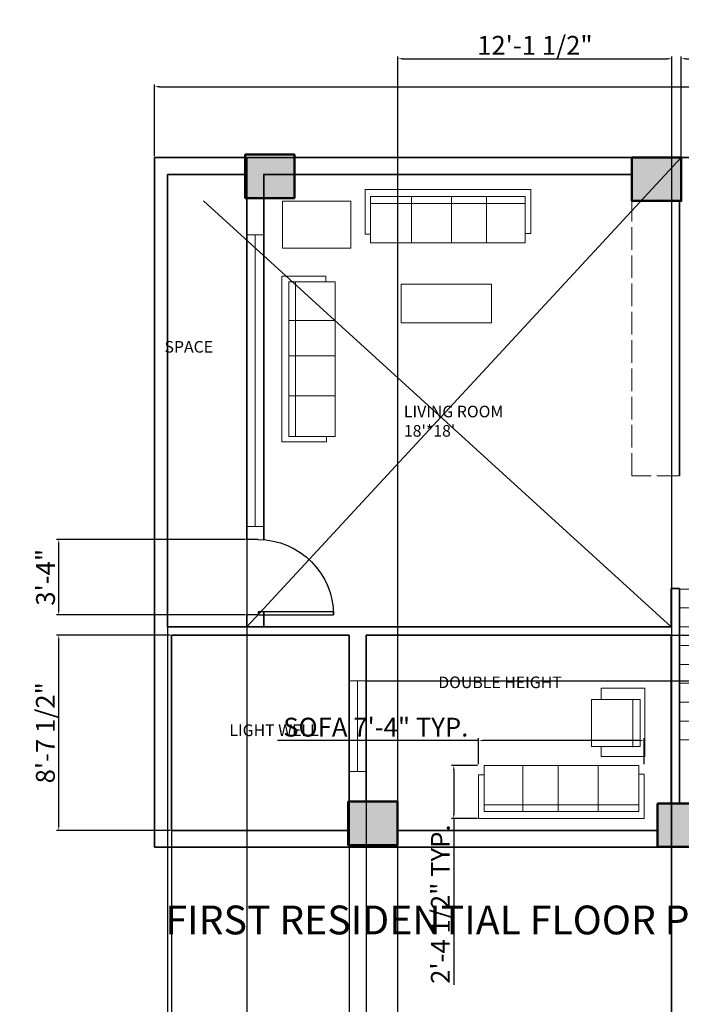
# Model space of a CAD drawing. Units: inches. Extents: x 1964 to 3462, y 1879 to 2909.
# Tile 3 of 4: x 2631 to 2982, y 2387 to 2909. Entities that reach past the tile are written whole.
import ezdxf

# ---------------------------------------------------------------- set-up
doc = ezdxf.new("R2010")
doc.units = ezdxf.units.IN
doc.linetypes.add('ACAD_ISO02W100', pattern=[15, 12, -3])
for name, color, linetype, lineweight in [('A-ANNO-DIMS', 2, 'Continuous', 18), ('A-ANNO-TEXT', 7, 'Continuous', 35), ('A-AREA-IDEN', 7, 'Continuous', 18), ('A-COLS', 1, 'Continuous', 50), ('A-COLS-PATT', 252, 'Continuous', 13), ('A-DOOR', 4, 'Continuous', 25), ('A-FLOR-OPEN', 8, 'Continuous', 13), ('A-FLOR-OVHD', 8, 'ACAD_ISO02W100', 18), ('A-FLOR-STRS', 3, 'Continuous', 18), ('A-FURN', 8, 'Continuous', 18), ('A-GLAZ', 4, 'Continuous', 18), ('A-WALL', 7, 'Continuous', 35)]:
    doc.layers.add(name, color=color, linetype=linetype, lineweight=lineweight)
doc.styles.get("Standard").update_dxf_attribs({"font": 'arial.ttf'})
doc.dimstyles.new('ISO-25', dxfattribs={"dimtxt": 10, "dimasz": 2.5, "dimexe": 1.25, "dimexo": 0.625, "dimtad": 1, "dimdec": 0, "dimlunit": 4, "dimtxsty": 'Standard', "dimcen": 2.5, "dimadec": 0, "dimazin": 0, "dimtfac": 1, "dimtdec": 0, "dimtmove": 0, "dimatfit": 3, "dimfxl": 1, "dimarcsym": 0})

# ---------------------------------------------------------------- blocks, each defined once
blk = doc.blocks.new('*U2')
for p, q in [((0, 0), (0, -6)), ((40, 0), (40, -6))]:
    blk.add_line(p, q)
blk.add_lwpolyline([(0, 0), (0, 40), (1.75, 40), (1.75, 0)], close=True)
blk.add_arc((0, 0), 40, 0, 90)
blk = doc.blocks.new('*D9')
at = {"layer": 'A-ANNO-DIMS', "color": 0, "lineweight": -2, "transparency": 16777216}
for p, q in [((2702.98, 2836.98), (2702.98, 2875.1)), ((2705.48, 2873.85), (3378.17, 2873.85)), ((3380.67, 2836.98), (3380.67, 2875.1))]:
    blk.add_line(p, q, dxfattribs=at)
at = {"layer": 'A-ANNO-DIMS', "color": 0, "lineweight": 100, "transparency": 16777216}
for points in [[(2705.48, 2874.26), (2705.48, 2873.43), (2702.98, 2873.85)], [(3378.17, 2874.26), (3378.17, 2873.43), (3380.67, 2873.85)]]:
    blk.add_solid(points, dxfattribs=at)
at = {"layer": 'Defpoints', "color": 0, "lineweight": 100, "transparency": 16777216}
for p in [(3380.67, 2873.85), (2702.98, 2836.36), (3380.67, 2836.36)]:
    blk.add_point(p, dxfattribs=at)
at = {"layer": 'A-ANNO-DIMS', "color": 0, "transparency": 16777216, "insert": (3041.82, 2879.58), "char_height": 10, "attachment_point": 5}
blk.add_mtext('56\'-6"', dxfattribs=at)
blk = doc.blocks.new('COL-RECT-26x23')
blk.add_lwpolyline([(0, 23.08), (26.15, 23.08), (26.15, 0), (0, 0)], close=True)
blk = doc.blocks.new('SOFA-4SEAT')
for p, q in [((0, 4.61), (0, 28.28)), ((0, 28.28), (87.86, 28.28)), ((87.86, 4.94), (87.86, 28.28)), ((2.86, 20.93), (84.86, 20.93)), ((24.5, 24.53), (24.5, 0)), ((45.74, 24.53), (45.74, 0)), ((64.36, 24.53), (64.36, 0)), ((2.86, 4.61), (0, 4.61)), ((84.86, 4.94), (87.86, 4.94))]:
    blk.add_line(p, q)
blk.add_lwpolyline([(2.86, 24.53), (84.86, 24.53), (84.86, 0), (2.86, 0)], close=True)
blk = doc.blocks.new('STAIR-RETURN-RESIDENTIAL')
for p, q in [((0, 128), (145.76, 128)), ((21.08, 128), (15.66, 121.5)), ((21.08, 21.87), (21.08, 128)), ((21.08, 128), (26.5, 121.5)), ((43.5, 124.05), (43.5, 128)), ((97.76, 128), (97.76, 118)), ((119.78, 128), (119.78, 21.87)), ((43.5, 48), (43.5, 124.05)), ((47.14, 51.64), (47.14, 120.41)), ((47.14, 120.41), (94.12, 120.41)), ((94.12, 51.64), (94.12, 120.41)), ((97.76, 48), (97.76, 124.05)), ((0, 118), (43.5, 118)), ((97.76, 118), (145.76, 118)), ((0, 108), (43.5, 108)), ((97.76, 108), (145.76, 108)), ((0, 98), (43.5, 98)), ((97.76, 98), (145.76, 98)), ((0, 88), (43.5, 88)), ((97.76, 88), (145.76, 88)), ((0, 78), (43.5, 78)), ((97.76, 78), (145.76, 78)), ((0, 68), (43.5, 68)), ((97.76, 68), (145.76, 68)), ((0, 58), (43.5, 58)), ((97.76, 58), (145.76, 58)), ((0, 48), (145.76, 48)), ((97.76, 48), (43.5, 48)), ((43.5, 48), (43.5, 0)), ((94.12, 51.64), (47.14, 51.64)), ((53.5, 48), (53.5, 0)), ((63.5, 48), (63.5, 0)), ((73.5, 48), (73.5, 0)), ((83.5, 48), (83.5, 0)), ((97.76, 50.18), (97.76, 0)), ((119.78, 21.87), (21.08, 21.87))]:
    blk.add_line(p, q)
blk = doc.blocks.new('WIN-48IN')
blk.add_line((4.5, 0), (4.5, 48.18))
blk.add_lwpolyline([(0, 0), (9, 0), (9, 48.18), (0, 48.18)], close=True)
blk = doc.blocks.new('*D25')
at = {"layer": 'A-ANNO-DIMS', "color": 0, "lineweight": -2, "transparency": 16777216}
for p, q in [((2874.86, 2514.46), (2874.86, 2528.27)), ((2962.72, 2514.46), (2962.72, 2528.27)), ((2874.86, 2527.02), (2768.29, 2527.02)), ((2960.22, 2527.02), (2877.36, 2527.02))]:
    blk.add_line(p, q, dxfattribs=at)
at = {"layer": 'A-ANNO-DIMS', "color": 0, "lineweight": 100, "transparency": 16777216}
for points in [[(2877.36, 2527.43), (2877.36, 2526.6), (2874.86, 2527.02)], [(2960.22, 2527.43), (2960.22, 2526.6), (2962.72, 2527.02)]]:
    blk.add_solid(points, dxfattribs=at)
at = {"layer": 'Defpoints', "color": 0, "lineweight": 100, "transparency": 16777216}
for p in [(2874.86, 2527.02), (2874.86, 2513.84), (2962.72, 2513.84)]:
    blk.add_point(p, dxfattribs=at)
at = {"layer": 'A-ANNO-DIMS', "color": 0, "transparency": 16777216, "insert": (2820.33, 2532.81), "char_height": 10, "attachment_point": 5}
blk.add_mtext('SOFA 7\'-4" TYP.', dxfattribs=at)
blk = doc.blocks.new('*D26')
at = {"layer": 'A-ANNO-DIMS', "color": 0, "lineweight": -2, "transparency": 16777216}
for p, q in [((2874.24, 2513.84), (2860.44, 2513.84)), ((2861.69, 2511.34), (2861.69, 2488.06)), ((2874.24, 2485.56), (2860.44, 2485.56)), ((2861.69, 2485.56), (2861.69, 2397.38))]:
    blk.add_line(p, q, dxfattribs=at)
at = {"layer": 'A-ANNO-DIMS', "color": 0, "lineweight": 100, "transparency": 16777216}
for points in [[(2861.27, 2511.34), (2862.1, 2511.34), (2861.69, 2513.84)], [(2861.27, 2488.06), (2862.1, 2488.06), (2861.69, 2485.56)]]:
    blk.add_solid(points, dxfattribs=at)
at = {"layer": 'Defpoints', "color": 0, "lineweight": 100, "transparency": 16777216}
for p in [(2874.86, 2513.84), (2861.69, 2485.56), (2874.86, 2485.56)]:
    blk.add_point(p, dxfattribs=at)
at = {"layer": 'A-ANNO-DIMS', "color": 0, "transparency": 16777216, "insert": (2855.89, 2440.22), "char_height": 10, "attachment_point": 5, "rotation": 90}
blk.add_mtext('2\'-4 1/2" TYP.', dxfattribs=at)
blk = doc.blocks.new('*D53')
at = {"layer": 'A-ANNO-DIMS', "color": 0, "lineweight": -2, "transparency": 16777216}
for p, q in [((2709.93, 2826.73), (2709.93, 1887.22)), ((2751.91, 2826.73), (2751.91, 1887.22)), ((2712.43, 1888.47), (2749.41, 1888.47))]:
    blk.add_line(p, q, dxfattribs=at)
at = {"layer": 'A-ANNO-DIMS', "color": 0, "lineweight": 100, "transparency": 16777216}
for points in [[(2712.43, 1888.89), (2712.43, 1888.06), (2709.93, 1888.47)], [(2749.41, 1888.89), (2749.41, 1888.06), (2751.91, 1888.47)]]:
    blk.add_solid(points, dxfattribs=at)
at = {"layer": 'Defpoints', "color": 0, "lineweight": 100, "transparency": 16777216}
for p in [(2709.93, 2827.36), (2751.91, 2827.36), (2751.91, 1888.47)]:
    blk.add_point(p, dxfattribs=at)
at = {"layer": 'A-ANNO-DIMS', "color": 0, "transparency": 16777216, "insert": (2730.92, 1894.21), "char_height": 10, "attachment_point": 5}
blk.add_mtext('3\'-6"', dxfattribs=at)
blk = doc.blocks.new('*D54')
at = {"layer": 'A-ANNO-DIMS', "color": 0, "lineweight": -2, "transparency": 16777216}
for p, q in [((2751.29, 2633.6), (2650.93, 2633.6)), ((2652.18, 2596.1), (2652.18, 2631.1)), ((2751.29, 2593.6), (2650.93, 2593.6))]:
    blk.add_line(p, q, dxfattribs=at)
at = {"layer": 'A-ANNO-DIMS', "color": 0, "lineweight": 100, "transparency": 16777216}
for points in [[(2651.76, 2631.1), (2652.59, 2631.1), (2652.18, 2633.6)], [(2651.76, 2596.1), (2652.59, 2596.1), (2652.18, 2593.6)]]:
    blk.add_solid(points, dxfattribs=at)
at = {"layer": 'Defpoints', "color": 0, "lineweight": 100, "transparency": 16777216}
for p in [(2652.18, 2633.6), (2751.91, 2633.6), (2751.91, 2593.6)]:
    blk.add_point(p, dxfattribs=at)
at = {"layer": 'A-ANNO-DIMS', "color": 0, "transparency": 16777216, "insert": (2646.44, 2613.6), "char_height": 10, "attachment_point": 5, "rotation": 90}
blk.add_mtext('3\'-4"', dxfattribs=at)
blk = doc.blocks.new('*D55')
at = {"layer": 'A-ANNO-DIMS', "color": 0, "lineweight": -2, "transparency": 16777216}
for p, q in [((2982.37, 2813.9), (2982.37, 2889.94)), ((2984.87, 2888.69), (3166.19, 2888.69)), ((3168.69, 2813.9), (3168.69, 2889.94))]:
    blk.add_line(p, q, dxfattribs=at)
at = {"layer": 'A-ANNO-DIMS', "color": 0, "lineweight": 100, "transparency": 16777216}
for points in [[(2984.87, 2889.1), (2984.87, 2888.27), (2982.37, 2888.69)], [(3166.19, 2889.1), (3166.19, 2888.27), (3168.69, 2888.69)]]:
    blk.add_solid(points, dxfattribs=at)
at = {"layer": 'Defpoints', "color": 0, "lineweight": 100, "transparency": 16777216}
for p in [(3168.69, 2888.69), (2982.37, 2813.28), (3168.69, 2813.28)]:
    blk.add_point(p, dxfattribs=at)
at = {"layer": 'A-ANNO-DIMS', "color": 0, "transparency": 16777216, "insert": (3075.53, 2894.48), "char_height": 10, "attachment_point": 5}
blk.add_mtext('15\'-6 1/2"', dxfattribs=at)
blk = doc.blocks.new('*D57')
at = {"layer": 'A-ANNO-DIMS', "color": 0, "lineweight": -2, "transparency": 16777216}
for p, q in [((2711.98, 2582.23), (2711.98, 1887.22)), ((2806.18, 2582.23), (2806.18, 1887.22)), ((2714.48, 1888.47), (2803.68, 1888.47))]:
    blk.add_line(p, q, dxfattribs=at)
at = {"layer": 'A-ANNO-DIMS', "color": 0, "lineweight": 100, "transparency": 16777216}
for points in [[(2714.48, 1888.89), (2714.48, 1888.06), (2711.98, 1888.47)], [(2803.68, 1888.89), (2803.68, 1888.06), (2806.18, 1888.47)]]:
    blk.add_solid(points, dxfattribs=at)
at = {"layer": 'Defpoints', "color": 0, "lineweight": 100, "transparency": 16777216}
for p in [(2711.98, 2582.86), (2806.18, 2582.86), (2806.18, 1888.47)]:
    blk.add_point(p, dxfattribs=at)
at = {"layer": 'A-ANNO-DIMS', "color": 0, "transparency": 16777216, "insert": (2759.08, 1894.2), "char_height": 10, "attachment_point": 5}
blk.add_mtext('7\'-10"', dxfattribs=at)
blk = doc.blocks.new('*D58')
at = {"layer": 'A-ANNO-DIMS', "color": 0, "lineweight": -2, "transparency": 16777216}
for p, q in [((2815.18, 2582.23), (2815.18, 1887.22)), ((2976.91, 2582.23), (2976.91, 1887.22)), ((2817.68, 1888.47), (2974.41, 1888.47))]:
    blk.add_line(p, q, dxfattribs=at)
at = {"layer": 'A-ANNO-DIMS', "color": 0, "lineweight": 100, "transparency": 16777216}
for points in [[(2817.68, 1888.89), (2817.68, 1888.06), (2815.18, 1888.47)], [(2974.41, 1888.89), (2974.41, 1888.06), (2976.91, 1888.47)]]:
    blk.add_solid(points, dxfattribs=at)
at = {"layer": 'Defpoints', "color": 0, "lineweight": 100, "transparency": 16777216}
for p in [(2815.18, 2582.86), (2976.91, 2582.86), (2976.91, 1888.47)]:
    blk.add_point(p, dxfattribs=at)
at = {"layer": 'A-ANNO-DIMS', "color": 0, "transparency": 16777216, "insert": (2896.05, 1894.27), "char_height": 10, "attachment_point": 5}
blk.add_mtext('13\'-5 1/2"', dxfattribs=at)
blk = doc.blocks.new('*D59')
at = {"layer": 'A-ANNO-DIMS', "color": 0, "lineweight": -2, "transparency": 16777216}
for p, q in [((2711.35, 2582.86), (2650.93, 2582.86)), ((2652.18, 2481.86), (2652.18, 2580.36)), ((2711.35, 2479.36), (2650.93, 2479.36))]:
    blk.add_line(p, q, dxfattribs=at)
at = {"layer": 'A-ANNO-DIMS', "color": 0, "lineweight": 100, "transparency": 16777216}
for points in [[(2651.76, 2580.36), (2652.59, 2580.36), (2652.18, 2582.86)], [(2651.76, 2481.86), (2652.59, 2481.86), (2652.18, 2479.36)]]:
    blk.add_solid(points, dxfattribs=at)
at = {"layer": 'Defpoints', "color": 0, "lineweight": 100, "transparency": 16777216}
for p in [(2652.18, 2582.86), (2711.98, 2582.86), (2711.98, 2479.36)]:
    blk.add_point(p, dxfattribs=at)
at = {"layer": 'A-ANNO-DIMS', "color": 0, "transparency": 16777216, "insert": (2646.38, 2531.11), "char_height": 10, "attachment_point": 5, "rotation": 90}
blk.add_mtext('8\'-7 1/2"', dxfattribs=at)
blk = doc.blocks.new('*D60')
at = {"layer": 'A-ANNO-DIMS', "color": 0, "lineweight": -2, "transparency": 16777216}
for p, q in [((3448.35, 2582.86), (3448.35, 2613.36)), ((2815.81, 2582.86), (3449.6, 2582.86)), ((3448.35, 2561.25), (3448.35, 2580.36)), ((2815.81, 2558.75), (3449.6, 2558.75))]:
    blk.add_line(p, q, dxfattribs=at)
at = {"layer": 'A-ANNO-DIMS', "color": 0, "lineweight": 100, "transparency": 16777216}
for points in [[(3447.94, 2580.36), (3448.77, 2580.36), (3448.35, 2582.86)], [(3447.94, 2561.25), (3448.77, 2561.25), (3448.35, 2558.75)]]:
    blk.add_solid(points, dxfattribs=at)
at = {"layer": 'Defpoints', "color": 0, "lineweight": 100, "transparency": 16777216}
for p in [(2815.18, 2582.86), (3448.35, 2582.86), (2815.18, 2558.75)]:
    blk.add_point(p, dxfattribs=at)
at = {"layer": 'A-ANNO-DIMS', "color": 0, "transparency": 16777216, "insert": (3442.62, 2599.36), "char_height": 10, "attachment_point": 5, "rotation": 90}
blk.add_mtext('2\'-0"', dxfattribs=at)
blk = doc.blocks.new('*D64')
at = {"layer": 'A-ANNO-DIMS', "color": 0, "lineweight": -2, "transparency": 16777216}
for p, q in [((2832.07, 2298.2), (2832.07, 2889.94)), ((2834.57, 2888.69), (2974.84, 2888.69)), ((2977.34, 2298.34), (2977.34, 2889.94))]:
    blk.add_line(p, q, dxfattribs=at)
at = {"layer": 'A-ANNO-DIMS', "color": 0, "lineweight": 100, "transparency": 16777216}
for points in [[(2834.57, 2889.1), (2834.57, 2888.27), (2832.07, 2888.69)], [(2974.84, 2889.1), (2974.84, 2888.27), (2977.34, 2888.69)]]:
    blk.add_solid(points, dxfattribs=at)
at = {"layer": 'Defpoints', "color": 0, "lineweight": 100, "transparency": 16777216}
for p in [(2977.34, 2888.69), (2832.07, 2297.57), (2977.34, 2297.71)]:
    blk.add_point(p, dxfattribs=at)
at = {"layer": 'A-ANNO-DIMS', "color": 0, "transparency": 16777216, "insert": (2904.7, 2894.48), "char_height": 10, "attachment_point": 5}
blk.add_mtext('12\'-1 1/2"', dxfattribs=at)

msp = doc.modelspace()

# ---------------------------------------------------------------- hatches: boundary and pattern name
at = {"layer": 'A-COLS-PATT'}
h = msp.add_hatch(color=256, dxfattribs=at)
h.dxf.hatch_style = 1
h.paths.add_polyline_path([(2777.22, 2827.36), (2760.91, 2827.36), (2760.91, 2814.8), (2777.22, 2814.8)], flags=17)
h.paths.add_polyline_path([(2777.22, 2836.36), (2751.91, 2836.36), (2751.91, 2814.8), (2760.91, 2814.8), (2760.91, 2827.36), (2777.22, 2827.36)])
h = msp.add_hatch(color=256, dxfattribs=at)
h.dxf.hatch_style = 1
h.paths.add_polyline_path([(3380.67, 2836.36), (3354.52, 2836.36), (3354.52, 2813.28), (3380.67, 2813.28)])
h.paths.add_polyline_path([(3194.85, 2836.36), (3168.69, 2836.36), (3168.69, 2827.36), (3168.91, 2827.36), (3168.91, 2813.28), (3194.85, 2813.28)])
h.paths.add_polyline_path([(2982.37, 2836.36), (2956.21, 2836.36), (2956.21, 2813.28), (2961, 2813.28)])
h.paths.add_polyline_path([(2982.37, 2836.36), (2961, 2813.28), (2981.41, 2813.28), (2982.37, 2813.28)], flags=17)
h.paths.add_polyline_path([(2831.78, 2494.67), (2805.62, 2494.67), (2805.62, 2471.58), (2831.78, 2471.58)])
h.paths.add_polyline_path([(2995.98, 2493.63), (2969.83, 2493.63), (2969.83, 2470.55), (2995.98, 2470.55)])
h.paths.add_polyline_path([(3252.83, 2493.16), (3226.67, 2493.16), (3226.67, 2470.36), (3252.83, 2470.36)])
h.paths.add_polyline_path([(3380.67, 2492.15), (3354.52, 2492.15), (3354.52, 2470.36), (3380.67, 2470.36)])

# ---------------------------------------------------------------- linework, layer by layer
at = {"layer": 'A-FLOR-OPEN'}
for p, q in [((2751.91, 2587.36), (2982.37, 2836.36)), ((2976.91, 2587.36), (2728.87, 2813.28))]:
    msp.add_line(p, q, dxfattribs=at)
at = {"layer": 'A-FLOR-OVHD'}
msp.add_lwpolyline([(2956.21, 2813.28), (2981.41, 2813.28), (2981.41, 2667.39), (2956.21, 2667.39)], close=True, dxfattribs=at)
at = {"layer": 'A-FURN'}
for p, q in [((2963, 2554.78), (2939.82, 2554.78)), ((2939.82, 2554.78), (2939.82, 2548.74)), ((2963, 2518.48), (2963, 2554.78)), ((2956.59, 2523.41), (2956.59, 2548.74)), ((2939.82, 2523.79), (2939.82, 2518.48)), ((2939.82, 2518.48), (2963, 2518.48))]:
    msp.add_line(p, q, dxfattribs=at)
for points in [[(2770.8, 2813.17), (2807.1, 2813.17), (2807.1, 2788.12), (2770.8, 2788.12)], [(2833.84, 2769.1), (2881.7, 2769.1), (2881.7, 2748.67), (2833.84, 2748.67)], [(2960.47, 2523.79), (2934.71, 2523.79), (2934.71, 2548.74), (2960.47, 2548.74)]]:
    msp.add_lwpolyline(points, close=True, dxfattribs=at)
at = {"layer": 'A-GLAZ'}
msp.add_line((2756.41, 2795.29), (2756.41, 2640.6), dxfattribs=at)
msp.add_lwpolyline([(2751.91, 2640.6), (2760.91, 2640.6), (2760.91, 2795.29), (2751.91, 2795.29)], close=True, dxfattribs=at)
at = {"layer": 'A-WALL'}
for p, q in [((2751.91, 2836.36), (2702.98, 2836.36)), ((2702.98, 2836.36), (2702.98, 2582.86)), ((2916.91, 2836.36), (2751.91, 2836.36)), ((2751.91, 2836.36), (2751.91, 2671.89)), ((2751.91, 2836.36), (2751.91, 2633.6)), ((2709.93, 2587.36), (2709.93, 2827.36)), ((2709.93, 2827.36), (2751.91, 2827.36)), ((2760.91, 2827.36), (2956.21, 2827.36)), ((2981.41, 2813.28), (2981.41, 2667.39)), ((2976.91, 2607.63), (2976.91, 2587.36)), ((2976.91, 2607.63), (2981.41, 2607.63)), ((2981.41, 2607.63), (2981.41, 2582.86)), ((2751.91, 2593.6), (2751.91, 2587.36)), ((2751.91, 2591.89), (2751.91, 2587.36)), ((2751.91, 2587.36), (2709.93, 2587.36)), ((2976.91, 2587.36), (2751.91, 2587.36)), ((2702.98, 2582.86), (2702.98, 2470.36)), ((2711.98, 2582.86), (2783.24, 2582.86)), ((2711.98, 2582.86), (2711.98, 2479.36)), ((2806.18, 2582.86), (2751.91, 2582.86)), ((2806.18, 2582.86), (2806.18, 2494.67)), ((2976.91, 2582.86), (2815.18, 2582.86)), ((2815.18, 2582.86), (2815.18, 2494.67)), ((2976.91, 2582.86), (2976.91, 2493.63)), ((2981.41, 2582.86), (2981.41, 2493.63)), ((2711.98, 2479.36), (2772.25, 2479.36)), ((2702.98, 2470.36), (2772.25, 2470.36)), ((2751.91, 2470.36), (2864.78, 2470.36))]:
    msp.add_line(p, q, dxfattribs=at)
for points in [[(2751.91, 2633.6), (2751.91, 2836.36), (3380.67, 2836.36), (3380.67, 2470.36), (2751.91, 2470.36)], [(3380.67, 2674.12), (3380.67, 2836.36), (2841.75, 2836.36)], [(2760.91, 2633.49), (2760.91, 2827.36), (2956.21, 2827.36)], [(2841.75, 2470.36), (3380.67, 2470.36), (3380.67, 2634.12)], [(2751.91, 2587.36), (2751.91, 2593.6)], [(2760.91, 2587.36), (2760.91, 2595.35)], [(2806.18, 2479.36), (2760.91, 2479.36)], [(2969.83, 2479.36), (2831.78, 2479.36)]]:
    msp.add_lwpolyline(points, dxfattribs=at)

# ---------------------------------------------------------------- block references
at = {"layer": 'A-COLS'}
for p in [(2751.06, 2814.8), (2956.21, 2813.28), (2805.62, 2471.58), (2969.83, 2470.55)]:
    msp.add_blockref('COL-RECT-26x23', p, dxfattribs=at)
at = {"layer": 'A-DOOR', "xscale": -1, "rotation": 270}
msp.add_blockref('*U2', (2757.91, 2593.6), dxfattribs=at)
at = {"layer": 'A-FLOR-STRS'}
msp.add_blockref('STAIR-RETURN-RESIDENTIAL', (2981.41, 2479.36), dxfattribs=at)
at = {"layer": 'A-FURN'}
msp.add_blockref('SOFA-4SEAT', (2814.69, 2790.99), dxfattribs=at)
for p, rotation in [((2798.76, 2685.4), 90.00000000000055), ((2962.72, 2513.84), 180)]:
    msp.add_blockref('SOFA-4SEAT', p, dxfattribs=dict(at, rotation=rotation))
at = {"layer": 'A-GLAZ'}
msp.add_blockref('WIN-48IN', (2806.18, 2510.57), dxfattribs=at)

# ---------------------------------------------------------------- texts
at = {"layer": 'A-ANNO-TEXT', "insert": (2708.78, 2439.45), "char_height": 15.2607, "attachment_point": 1}
msp.add_mtext_dynamic_manual_height_columns('FIRST RESIDENTIAL FLOOR PLAN', width=480.7827, gutter_width=76.3, heights=[0], dxfattribs=at)
at = {"layer": 'A-AREA-IDEN', "attachment_point": 1}
for s, insert, char_height in [('SPACE', (2708.28, 2738.94), 6.161), ("LIVING ROOM\\P18'*18'", (2835.24, 2704.62), 6.1611), ('DOUBLE HEIGHT', (2853.47, 2560.97), 6.1611), ('LIGHT WELL', (2742.71, 2535.54), 6.161)]:
    msp.add_mtext_dynamic_manual_height_columns(s, width=194.1034, gutter_width=30.81, heights=[0], dxfattribs=dict(at, insert=insert, char_height=char_height))

# ---------------------------------------------------------------- dimensions: what is measured, and where the dimension line sits
at = {"layer": 'A-ANNO-DIMS'}
for base, p1, p2, override, picture, middle in [((2977.34, 2888.69), (2832.07, 2297.57), (2977.34, 2297.71), {"dimdec": 1, "dimlfac": 1, "dimrnd": 0, "dimzin": 1, "dimdsep": 46, "dimlunit": 4, "dimfrac": 2}, '*D64', (2904.7, 2894.48)), ((3168.69, 2888.69), (2982.37, 2813.28), (3168.69, 2813.28), {"dimdec": 1, "dimlfac": 1, "dimrnd": 0, "dimzin": 1, "dimdsep": 46, "dimlunit": 4, "dimfrac": 2}, '*D55', (3075.53, 2894.48)), ((3380.67, 2873.85), (2702.98, 2836.36), (3380.67, 2836.36), {"dimclrd": 0, "dimclre": 0, "dimclrt": 0}, '*D9', (3041.82, 2879.58)), ((2751.91, 1888.47), (2709.93, 2827.36), (2751.91, 2827.36), {"dimdec": 1, "dimlfac": 1, "dimrnd": 0, "dimzin": 1, "dimdsep": 46, "dimlunit": 4, "dimfrac": 2}, '*D53', (2730.92, 1894.21)), ((2806.18, 1888.47), (2711.98, 2582.86), (2806.18, 2582.86), {"dimdec": 1, "dimlfac": 1, "dimrnd": 0, "dimzin": 1, "dimdsep": 46, "dimlunit": 4, "dimfrac": 2}, '*D57', (2759.08, 1894.2)), ((2976.91, 1888.47), (2815.18, 2582.86), (2976.91, 2582.86), {"dimdec": 1, "dimlfac": 1, "dimrnd": 0, "dimzin": 1, "dimdsep": 46, "dimlunit": 4, "dimfrac": 2}, '*D58', (2896.05, 1894.27))]:
    dim = msp.add_linear_dim(base=base, p1=p1, p2=p2, dimstyle='ISO-25', override=override, dxfattribs=at)
    dim.commit()
    dim.dimension.update_dxf_attribs({"geometry": picture, "text_midpoint": middle})
for base, p1, p2, picture, middle in [((2652.18, 2633.6), (2751.91, 2593.6), (2751.91, 2633.6), '*D54', (2646.44, 2613.6)), ((3448.35, 2582.86), (2815.18, 2558.75), (2815.18, 2582.86), '*D60', (3442.62, 2599.36)), ((2652.18, 2582.86), (2711.98, 2479.36), (2711.98, 2582.86), '*D59', (2646.38, 2531.11))]:
    dim = msp.add_linear_dim(base=base, p1=p1, p2=p2, angle=90, dimstyle='ISO-25', override={"dimdec": 1, "dimlfac": 1, "dimrnd": 0, "dimzin": 1, "dimdsep": 46, "dimlunit": 4, "dimfrac": 2}, dxfattribs=at)
    dim.commit()
    dim.dimension.update_dxf_attribs({"geometry": picture, "text_midpoint": middle})
for base, p1, p2, angle, text, picture, middle in [((2874.86, 2527.02), (2962.72, 2513.84), (2874.86, 2513.84), 180, 'SOFA <> TYP.', '*D25', (2820.33, 2532.81)), ((2861.69, 2485.56), (2874.86, 2513.84), (2874.86, 2485.56), 270, '<> TYP.', '*D26', (2855.89, 2440.22))]:
    dim = msp.add_linear_dim(base=base, p1=p1, p2=p2, angle=angle, text=text, dimstyle='ISO-25', override={"dimdec": 1, "dimlfac": 1, "dimrnd": 0, "dimzin": 1, "dimdsep": 46, "dimlunit": 4, "dimfrac": 2}, dxfattribs=at)
    dim.commit()
    dim.dimension.update_dxf_attribs({"geometry": picture, "text_midpoint": middle})

doc.saveas('drawing.dxf')
